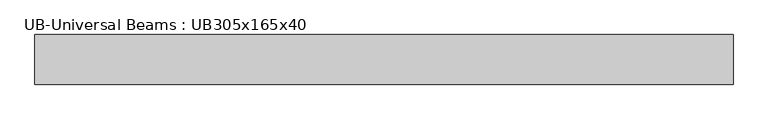
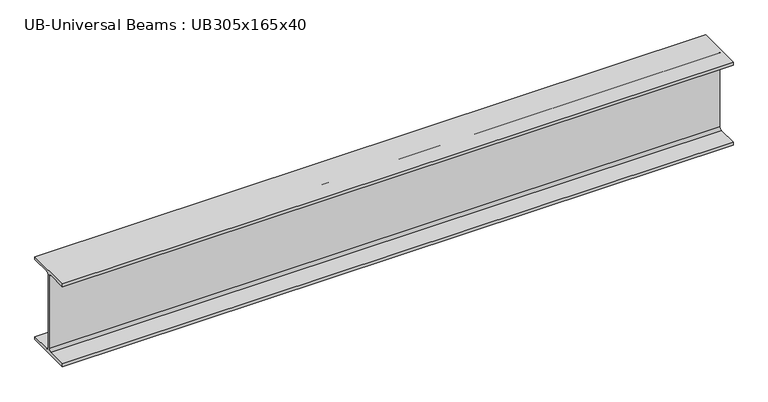
"""IFC4 building model written with IfcOpenShell, lengths in millimetres: beam geometry, UB-Universal Beams : UB305x165x40."""

from ifc_helpers import new_model, si_unit, point, frame, frame_2d, origin, place, context, project, spatial, polyline, circle_curve, trimmed, segment, composite_curve, outline, extrude, source, transform, mapped, element, save


def ub_universal_beams_ub305x165x40_dcb3c2ea(model_context):
    return source(origin(), model_context, "Body", "SweptSolid", [
        extrude(outline(composite_curve([segment(polyline([(82.5, -141.5), (82.5, -151.7), (-82.5, -151.7), (-82.5, -141.5), (-11.9, -141.5)]), True, "CONTINUOUS"), segment(trimmed(circle_curve(frame_2d((-11.9, -132.6)), 8.9), [point((-11.9, -141.5))], [point((-3.0, -132.6))], True, "CARTESIAN"), True, "CONTINUOUS"), segment(polyline([(-3.0, -132.6), (-3.0, 132.6)]), True, "CONTINUOUS"), segment(trimmed(circle_curve(frame_2d((-11.9, 132.6)), 8.9), [point((-3.0, 132.6))], [point((-11.9, 141.5))], True, "CARTESIAN"), True, "CONTINUOUS"), segment(polyline([(-11.9, 141.5), (-82.5, 141.5), (-82.5, 151.7), (82.5, 151.7), (82.5, 141.5), (11.9, 141.5)]), True, "CONTINUOUS"), segment(trimmed(circle_curve(frame_2d((11.9, 132.6)), 8.9), [point((11.9, 141.5))], [point((3.0, 132.6))], True, "CARTESIAN"), True, "CONTINUOUS"), segment(polyline([(3.0, 132.6), (3.0, -132.6)]), True, "CONTINUOUS"), segment(trimmed(circle_curve(frame_2d((11.9, -132.6)), 8.9), [point((3.0, -132.6))], [point((11.9, -141.5))], True, "CARTESIAN"), True, "CONTINUOUS"), segment(polyline([(11.9, -141.5), (82.5, -141.5)]), True, "CONTINUOUS")], self_intersect=False)), frame((-1093.1, 0.0, 0.0), z_axis=(1.0, 0.0, 0.0), x_axis=(0.0, 1.0, 0.0)), (0.0, 0.0, 1.0), 2323.0),
    ])


if __name__ == "__main__":
    model = new_model("IFC4")
    model_context = context("Model", 3, world=origin())
    ifc_project = project(units=[si_unit("LENGTHUNIT", "METRE", prefix="MILLI")], contexts=[model_context])
    site = spatial("IfcSite", under=ifc_project)
    building = spatial("IfcBuilding", under=site)
    placement = place(None, origin())
    ub_universal_beams_ub305x165x40_shape = ub_universal_beams_ub305x165x40_dcb3c2ea(model_context)
    element("IfcBeam", 1, ObjectType="UB-Universal Beams : UB305x165x40", at=placement, inside=building, context=model_context, shape_type="MappedRepresentation", body=[
        mapped(ub_universal_beams_ub305x165x40_shape, transform((0.0, 0.0, 0.0), x_axis=(1.0, 0.0, 0.0), y_axis=(0.0, 1.0, 0.0), z_axis=(0.0, 0.0, 1.0))),
    ])
    save(model, "model.ifc")

# Revit data of these elements
# Type "UB-Universal Beams : UB305x165x40"
#   Section Name Key = "UB305X165X40"
#   Width = 16.5 cm
#   Web Thickness = 0.6 cm
#   Web Fillet = 0.89 cm
#   Warping Constant = 164000.0 cm⁶
#   Torsional Moment of Inertia = 14.70 cm⁴
#   Section Area = 51.3 cm²
#   Plastic Modulus weak axis = 142.0 cm³
#   Plastic Modulus strong axis = 623.0 cm³
#   Nominal Weight = 40.2999 kgf/m
#   Moment of Inertia weak axis = 764.00 cm⁴
#   Moment of Inertia strong axis = 8503.00 cm⁴
#   Height = 30.34 cm
#   Flange Thickness = 1.02 cm
#   Elastic Modulus weak axis = 92.6 cm³
#   Elastic Modulus strong axis = 560.0 cm³
#   Centroid Vertical = 15.17 cm
#   Centroid Horizontal = 8.25 cm
#   Bolt Spacing = 9.0 cm
#   Length [instance default] = 1500 mm
#   Structural Material [instance default] = Metal - Steel 43-275
#   Type Comments = ""
#   Assembly Code = ""
# Element 1 (IfcBeam, "UB-Universal Beams : UB305x165x40")
#   Materials on its faces: "Metal - Steel 43-275"
# Materials
#   "Metal - Steel 43-275": class "Metal", colour RGB 247 247 247, transparency 0, Cost = 0
